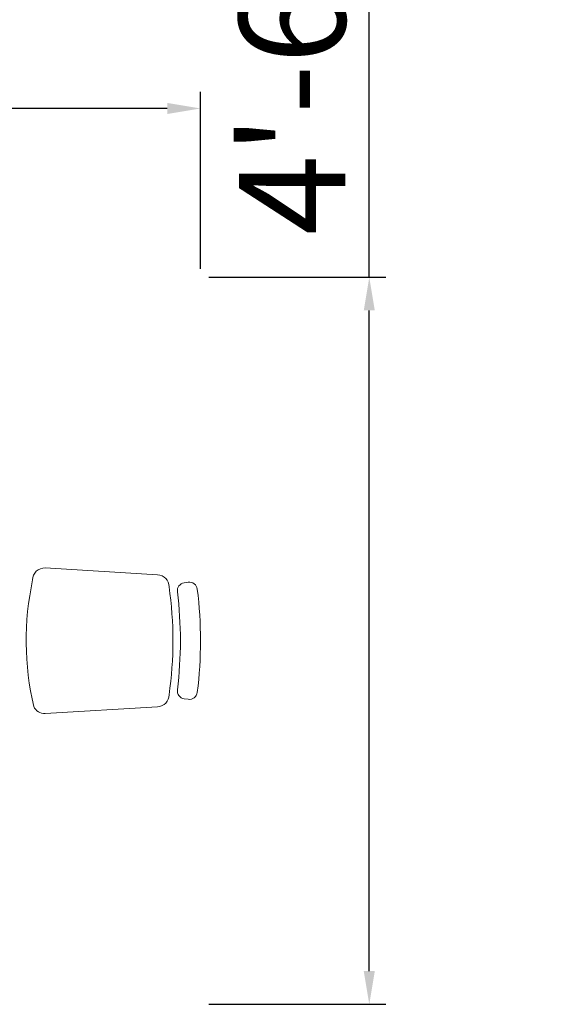
# Model space of a CAD drawing. Units: inches. Extents: x 1913 to 5309, y 1003 to 1733.
# Tile 19 of 23: x 4275 to 4315, y 1415 to 1489. Entities that reach past the tile are written whole.
import ezdxf

# ---------------------------------------------------------------- set-up
doc = ezdxf.new("R2010")
doc.units = ezdxf.units.IN
doc.layers.add('A-ANNO-DIMS', color=2, linetype='Continuous', lineweight=18)
doc.layers.add('A-FURN', color=8, linetype='Continuous', lineweight=18)
doc.styles.get("Standard").update_dxf_attribs({"font": 'arial.ttf'})
doc.dimstyles.new('ISO-25', dxfattribs={"dimtxt": 8, "dimasz": 2.5, "dimexe": 1.25, "dimexo": 0.625, "dimtad": 1, "dimdec": 1, "dimlunit": 3, "dimtxsty": 'Standard', "dimcen": 2.5, "dimclrd": 256, "dimclrt": 1, "dimadec": 0, "dimazin": 0, "dimtfac": 1, "dimtdec": 1, "dimtmove": 0, "dimatfit": 3, "dimfxl": 1, "dimarcsym": 0})

# ---------------------------------------------------------------- blocks, each defined once
blk = doc.blocks.new('A$C421907B3')
at = {"ltscale": 0.1}
for points in [[(0.77, 0.0782, -0.399285), (0.74, 0.1067), (0.7231, 0.3861, -0.305593), (0.7404, 0.4148, -0.109362), (1.0554, 0.4176, -0.429301), (1.0853, 0.3861), (1.0684, 0.1067, -0.399285), (1.0384, 0.0782, -0.071734)], [(0.9042, 0.05, 0.030867), (1.0261, 0.0575, -0.408428), (1.0484, 0.0405), (1.0498, 0.0306, -0.419966), (1.0325, 0.0079, -0.030916), (0.9042, 0, -0.030916), (0.7759, 0.0079, -0.419966), (0.7586, 0.0306), (0.76, 0.0405, -0.408428), (0.7823, 0.0575, 0.030867)]]:
    blk.add_lwpolyline(points, format="xyb", close=True, dxfattribs=at)
blk = doc.blocks.new('*D83')
at = {"layer": 'A-ANNO-DIMS', "color": 0, "lineweight": -2, "transparency": 16777216}
for p, q in [((4203.554, 1470.026), (4203.554, 1483.351)), ((4288.218, 1470.026), (4288.218, 1483.351))]:
    blk.add_line(p, q, dxfattribs=at)
at = {"layer": 'A-ANNO-DIMS', "lineweight": -2, "transparency": 16777216}
for p, q in [((4203.554, 1482.101), (4065.736, 1482.101)), ((4285.718, 1482.101), (4206.054, 1482.101))]:
    blk.add_line(p, q, dxfattribs=at)
at = {"layer": 'A-ANNO-DIMS', "transparency": 16777216}
for points in [[(4206.054, 1482.518), (4206.054, 1481.684), (4203.554, 1482.101)], [(4285.718, 1482.518), (4285.718, 1481.684), (4288.218, 1482.101)]]:
    blk.add_solid(points, dxfattribs=at)
at = {"layer": 'Defpoints', "color": 0, "transparency": 16777216}
for p in [(4203.554, 1482.101), (4203.554, 1469.401), (4288.218, 1469.401)]:
    blk.add_point(p, dxfattribs=at)
at = {"layer": 'A-ANNO-DIMS', "color": 1, "transparency": 16777216, "insert": (4133.395, 1486.862), "char_height": 8, "attachment_point": 5}
blk.add_mtext('DINING SET 7\'-0 1/2" TYP.', dxfattribs=at)
blk = doc.blocks.new('*D84')
at = {"layer": 'A-ANNO-DIMS', "lineweight": -2, "transparency": 16777216}
for p, q in [((4300.918, 1469.401), (4300.918, 1540.879)), ((4300.918, 1417.178), (4300.918, 1466.901))]:
    blk.add_line(p, q, dxfattribs=at)
at = {"layer": 'A-ANNO-DIMS', "color": 0, "lineweight": -2, "transparency": 16777216}
for p, q in [((4288.843, 1469.401), (4302.168, 1469.401)), ((4288.843, 1414.678), (4302.168, 1414.678))]:
    blk.add_line(p, q, dxfattribs=at)
at = {"layer": 'A-ANNO-DIMS', "transparency": 16777216}
for points in [[(4300.501, 1466.901), (4301.334, 1466.901), (4300.918, 1469.401)], [(4300.501, 1417.178), (4301.334, 1417.178), (4300.918, 1414.678)]]:
    blk.add_solid(points, dxfattribs=at)
at = {"layer": 'Defpoints', "color": 0, "transparency": 16777216}
for p in [(4288.218, 1469.401), (4300.918, 1469.401), (4288.218, 1414.678)]:
    blk.add_point(p, dxfattribs=at)
at = {"layer": 'A-ANNO-DIMS', "color": 1, "transparency": 16777216, "insert": (4296.156, 1506.39), "char_height": 8, "attachment_point": 5, "rotation": 90}
blk.add_mtext('4\'-6 1/2" TYP.', dxfattribs=at)

msp = doc.modelspace()

# ---------------------------------------------------------------- block references
at = {"layer": 'A-FURN', "xscale": 30.26057373645948, "yscale": 30.26057373645948, "zscale": 30.26057373645948, "rotation": 89.99999999999996}
msp.add_blockref('A$C421907B3', (4288.218, 1414.678), dxfattribs=at)

# ---------------------------------------------------------------- dimensions: what is measured, and where the dimension line sits
at = {"layer": 'A-ANNO-DIMS'}
for base, p1, p2, angle, text, picture, middle in [((4300.918, 1469.401), (4288.218, 1414.678), (4288.218, 1469.401), 90, '<> TYP.', '*D84', (4296.156, 1506.39)), ((4203.554, 1482.101), (4288.218, 1469.401), (4203.554, 1469.401), 180, 'DINING SET <> TYP.', '*D83', (4133.395, 1486.862))]:
    dim = msp.add_linear_dim(base=base, p1=p1, p2=p2, angle=angle, text=text, dimstyle='ISO-25', override={"dimdec": 1, "dimrnd": 0, "dimzin": 1, "dimlunit": 4, "dimfrac": 2}, dxfattribs=at)
    dim.commit()
    dim.dimension.update_dxf_attribs({"geometry": picture, "text_midpoint": middle})

doc.saveas('drawing.dxf')
